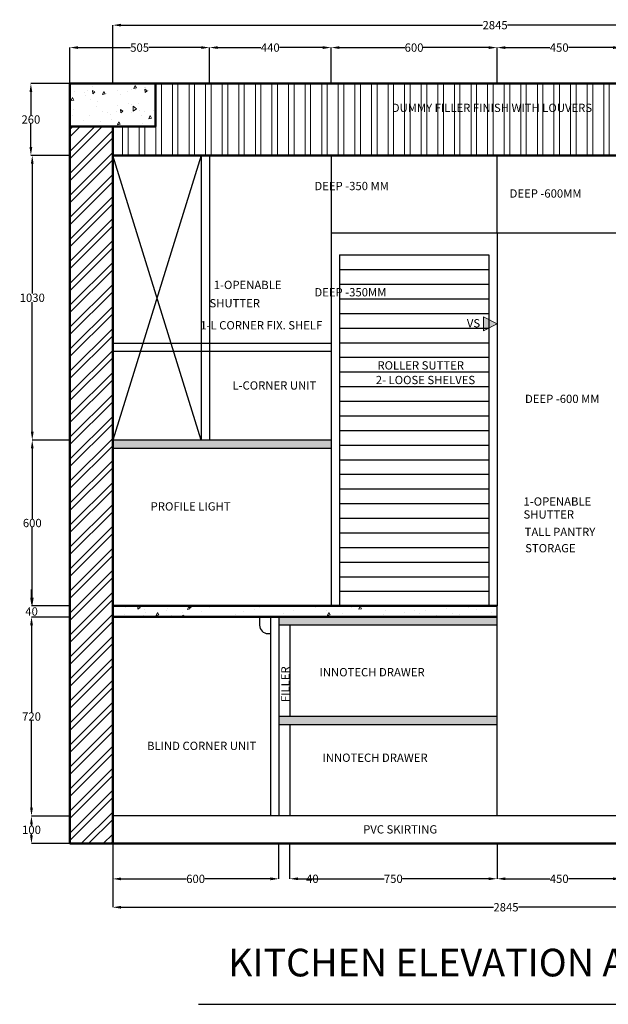
# Model space of a CAD drawing. Units: millimetres. Extents: x 26138 to 44889, y 15820 to 21179.
# Tile 7 of 8: x 41289 to 43418, y 15893 to 19455. Entities that reach past the tile are written whole.
import ezdxf

# ---------------------------------------------------------------- set-up
doc = ezdxf.new("R2010")
doc.units = ezdxf.units.MM
doc.header["$MEASUREMENT"] = 0
doc.header["$PDMODE"] = 3
for name, color, linetype, lineweight in [('A-ANNO-DIMS', 70, 'Continuous', 18), ('A-ANNO-SYMB', 1, 'Continuous', 18), ('A-ANNO-TEXT', 7, 'Continuous', 18), ('A-ELEV', 7, 'Continuous', 25), ('A-FURN-PATT', 40, 'Continuous', 13), ('A-WALL', 1, 'Continuous', 50), ('A-WALL-PATT', 8, 'Continuous', 13)]:
    doc.layers.add(name, color=color, linetype=linetype, lineweight=lineweight)
doc.styles.get("Standard").update_dxf_attribs({"font": 'arial.ttf'})
doc.dimstyles.get("Standard").update_dxf_attribs({"dimtxt": 30, "dimasz": 30, "dimexe": 0.18, "dimexo": 0.0625, "dimgap": 0.09, "dimtad": 0, "dimtih": 1, "dimtoh": 1, "dimdec": 0, "dimzin": 0, "dimdsep": 46, "dimtxsty": 'Standard', "dimcen": 0.09, "dimadec": 0, "dimazin": 0, "dimtfac": 1, "dimtdec": 0, "dimtofl": 0, "dimtmove": 0, "dimatfit": 3, "dimfxl": 1, "dimtolj": 1, "dimtzin": 0, "dimarcsym": 0})
pattern_1 = [(95, (-2438.25, -2020.09), (88.24832, 74.04913), [12, -132]), (40, (-2438.25, -2020.09), (-100.79875, 69.4029), [9.6, -105.6]), (145.45144, (-2430.9, -2013.92), (-12.55043, 143.45204), [10.19843, -112.18274]), (91.1842, (-2460.88, -1997.47), (139.47094, 102.0182), [18, -198]), (141.63564, (-2449.26, -1988.96), (-4.464, 215.95387), [15.29765, -168.2742]), (36.18416, (-2460.88, -1997.47), (-4.464, 215.95387), [14.4, -158.4]), (66, (-2443.91, -1991.81), (113.08345, 21.9812), [12, -132]), (11, (-2443.91, -1991.81), (-54.51337, 109.56935), [9.6, -105.6]), (116.45144, (-2434.49, -1989.98), (58.57008, 131.55054), [10.19843, -112.18274]), (82.5, (-2438.253, -2020.094), (-36.28691, 39.03837), [0, -104.32, 0, -107.2, 0, -106]), (52.5, (-2438.253, -2020.094), (-14.85967, 74.38551), [0, -61.12, 0, -101.92, 0, -40.4]), (12.5, (-2463.483, -2045.323), (62.946907, 57.843322), [0, -40, 0, -124.8, 0, -165.6]), (2.5, (-2474.796, -2056.64), (54.6544, 77.30557), [0, -52, 0, -82.88, 0, -117.6])]

# ---------------------------------------------------------------- blocks, each defined once
blk = doc.blocks.new('*D93')
at = {"layer": 'A-ANNO-DIMS', "color": 0, "lineweight": -2, "transparency": 16777216}
for p, q in [((41470.8, 19224.3), (41470.8, 19354.6)), ((41500.8, 19354.4), (41690, 19354.4)), ((41945.8, 19354.4), (41756.6, 19354.4)), ((41975.8, 19224.3), (41975.8, 19354.6))]:
    blk.add_line(p, q, dxfattribs=at)
at = {"layer": 'A-ANNO-DIMS', "color": 0, "transparency": 16777216}
for points in [[(41500.8, 19359.4), (41500.8, 19349.4), (41470.8, 19354.4)], [(41945.8, 19359.4), (41945.8, 19349.4), (41975.8, 19354.4)]]:
    blk.add_solid(points, dxfattribs=at)
at = {"layer": 'Defpoints', "color": 0, "transparency": 16777216}
for p in [(41975.8, 19354.4), (41470.8, 19224.2), (41975.8, 19224.2)]:
    blk.add_point(p, dxfattribs=at)
at = {"layer": 'A-ANNO-DIMS', "color": 0, "transparency": 16777216, "insert": (41723.3, 19354.4), "char_height": 30, "attachment_point": 5}
blk.add_mtext('\\A1;505', dxfattribs=at)
blk = doc.blocks.new('*D94')
at = {"layer": 'A-ANNO-DIMS', "color": 0, "lineweight": -2, "transparency": 16777216}
for p, q in [((41975.8, 19224.3), (41975.8, 19354.6)), ((42005.8, 19354.4), (42162, 19354.4)), ((42385.8, 19354.4), (42229.6, 19354.4)), ((42415.8, 19224.3), (42415.8, 19354.6))]:
    blk.add_line(p, q, dxfattribs=at)
at = {"layer": 'A-ANNO-DIMS', "color": 0, "transparency": 16777216}
for points in [[(42005.8, 19359.4), (42005.8, 19349.4), (41975.8, 19354.4)], [(42385.8, 19359.4), (42385.8, 19349.4), (42415.8, 19354.4)]]:
    blk.add_solid(points, dxfattribs=at)
at = {"layer": 'Defpoints', "color": 0, "transparency": 16777216}
for p in [(42415.8, 19354.4), (41975.8, 19224.2), (42415.8, 19224.2)]:
    blk.add_point(p, dxfattribs=at)
at = {"layer": 'A-ANNO-DIMS', "color": 0, "transparency": 16777216, "insert": (42195.8, 19354.4), "char_height": 30, "attachment_point": 5}
blk.add_mtext('\\A1;440', dxfattribs=at)
blk = doc.blocks.new('*D95')
at = {"layer": 'A-ANNO-DIMS', "color": 0, "lineweight": -2, "transparency": 16777216}
for p, q in [((42415.8, 19224.3), (42415.8, 19354.6)), ((42445.8, 19354.4), (42682.5, 19354.4)), ((42985.8, 19354.4), (42749.1, 19354.4)), ((43015.8, 19224.3), (43015.8, 19354.6))]:
    blk.add_line(p, q, dxfattribs=at)
at = {"layer": 'A-ANNO-DIMS', "color": 0, "transparency": 16777216}
for points in [[(42445.8, 19359.4), (42445.8, 19349.4), (42415.8, 19354.4)], [(42985.8, 19359.4), (42985.8, 19349.4), (43015.8, 19354.4)]]:
    blk.add_solid(points, dxfattribs=at)
at = {"layer": 'Defpoints', "color": 0, "transparency": 16777216}
for p in [(43015.8, 19354.4), (42415.8, 19224.2), (43015.8, 19224.2)]:
    blk.add_point(p, dxfattribs=at)
at = {"layer": 'A-ANNO-DIMS', "color": 0, "transparency": 16777216, "insert": (42715.8, 19354.4), "char_height": 30, "attachment_point": 5}
blk.add_mtext('\\A1;600', dxfattribs=at)
blk = doc.blocks.new('*D96')
at = {"layer": 'A-ANNO-DIMS', "color": 0, "lineweight": -2, "transparency": 16777216}
for p, q in [((43015.8, 19224.3), (43015.8, 19354.6)), ((43045.8, 19354.4), (43207, 19354.4)), ((43435.8, 19354.4), (43274.6, 19354.4)), ((43465.8, 19224.3), (43465.8, 19354.6))]:
    blk.add_line(p, q, dxfattribs=at)
at = {"layer": 'A-ANNO-DIMS', "color": 0, "transparency": 16777216}
for points in [[(43045.8, 19359.4), (43045.8, 19349.4), (43015.8, 19354.4)], [(43435.8, 19359.4), (43435.8, 19349.4), (43465.8, 19354.4)]]:
    blk.add_solid(points, dxfattribs=at)
at = {"layer": 'Defpoints', "color": 0, "transparency": 16777216}
for p in [(43465.8, 19354.4), (43015.8, 19224.2), (43465.8, 19224.2)]:
    blk.add_point(p, dxfattribs=at)
at = {"layer": 'A-ANNO-DIMS', "color": 0, "transparency": 16777216, "insert": (43240.8, 19354.4), "char_height": 30, "attachment_point": 5}
blk.add_mtext('\\A1;450', dxfattribs=at)
blk = doc.blocks.new('*D99')
at = {"layer": 'A-ANNO-DIMS', "color": 0, "lineweight": -2, "transparency": 16777216}
for p, q in [((41625.8, 19224.3), (41625.8, 19435.8)), ((41655.8, 19435.6), (42963.6, 19435.6)), ((44440.8, 19435.6), (43054.1, 19435.6)), ((44470.8, 19224.3), (44470.8, 19435.8))]:
    blk.add_line(p, q, dxfattribs=at)
at = {"layer": 'A-ANNO-DIMS', "color": 0, "transparency": 16777216}
for points in [[(41655.8, 19440.6), (41655.8, 19430.6), (41625.8, 19435.6)], [(44440.8, 19440.6), (44440.8, 19430.6), (44470.8, 19435.6)]]:
    blk.add_solid(points, dxfattribs=at)
at = {"layer": 'Defpoints', "color": 0, "transparency": 16777216}
for p in [(41625.8, 19435.6), (41625.8, 19224.2), (44470.8, 19224.2)]:
    blk.add_point(p, dxfattribs=at)
at = {"layer": 'A-ANNO-DIMS', "color": 0, "transparency": 16777216, "insert": (43008.9, 19435.6), "char_height": 30, "attachment_point": 5}
blk.add_mtext('\\A1;2845', dxfattribs=at)
blk = doc.blocks.new('*D105')
at = {"layer": 'A-ANNO-DIMS', "color": 0, "lineweight": -2, "transparency": 16777216}
for p, q in [((41625.8, 16474.2), (41625.8, 16346.6)), ((42225.8, 16474.2), (42225.8, 16346.6)), ((41655.8, 16346.7), (41892.5, 16346.7)), ((42195.8, 16346.7), (41959.1, 16346.7))]:
    blk.add_line(p, q, dxfattribs=at)
at = {"layer": 'A-ANNO-DIMS', "color": 0, "transparency": 16777216}
for points in [[(41655.8, 16351.7), (41655.8, 16341.7), (41625.8, 16346.7)], [(42195.8, 16351.7), (42195.8, 16341.7), (42225.8, 16346.7)]]:
    blk.add_solid(points, dxfattribs=at)
at = {"layer": 'Defpoints', "color": 0, "transparency": 16777216}
for p in [(41625.8, 16474.2), (42225.8, 16474.2), (42225.8, 16346.7)]:
    blk.add_point(p, dxfattribs=at)
at = {"layer": 'A-ANNO-DIMS', "color": 0, "transparency": 16777216, "insert": (41925.8, 16346.7), "char_height": 30, "attachment_point": 5}
blk.add_mtext('\\A1;600', dxfattribs=at)
blk = doc.blocks.new('*D106')
at = {"layer": 'A-ANNO-DIMS', "color": 0, "lineweight": -2, "transparency": 16777216}
for p, q in [((42225.8, 16474.2), (42225.8, 16346.9)), ((42265.8, 16474.2), (42265.8, 16346.9)), ((42195.8, 16347.1), (42165.8, 16347.1)), ((42295.8, 16347.1), (42325.8, 16347.1))]:
    blk.add_line(p, q, dxfattribs=at)
at = {"layer": 'A-ANNO-DIMS', "color": 0, "transparency": 16777216}
for points in [[(42195.8, 16352.1), (42195.8, 16342.1), (42225.8, 16347.1)], [(42295.8, 16352.1), (42295.8, 16342.1), (42265.8, 16347.1)]]:
    blk.add_solid(points, dxfattribs=at)
at = {"layer": 'Defpoints', "color": 0, "transparency": 16777216}
for p in [(42225.8, 16474.2), (42265.8, 16474.2), (42265.8, 16347.1)]:
    blk.add_point(p, dxfattribs=at)
at = {"layer": 'A-ANNO-DIMS', "color": 0, "transparency": 16777216, "insert": (42347.9, 16347.1), "char_height": 30, "attachment_point": 5}
blk.add_mtext('\\A1;40', dxfattribs=at)
blk = doc.blocks.new('*D107')
at = {"layer": 'A-ANNO-DIMS', "color": 0, "lineweight": -2, "transparency": 16777216}
for p, q in [((42265.8, 16474.2), (42265.8, 16346.9)), ((43015.8, 16474.2), (43015.8, 16346.9)), ((42295.8, 16347.1), (42607.7, 16347.1)), ((42985.8, 16347.1), (42673.9, 16347.1))]:
    blk.add_line(p, q, dxfattribs=at)
at = {"layer": 'A-ANNO-DIMS', "color": 0, "transparency": 16777216}
for points in [[(42295.8, 16352.1), (42295.8, 16342.1), (42265.8, 16347.1)], [(42985.8, 16352.1), (42985.8, 16342.1), (43015.8, 16347.1)]]:
    blk.add_solid(points, dxfattribs=at)
at = {"layer": 'Defpoints', "color": 0, "transparency": 16777216}
for p in [(42265.8, 16474.2), (43015.8, 16474.2), (43015.8, 16347.1)]:
    blk.add_point(p, dxfattribs=at)
at = {"layer": 'A-ANNO-DIMS', "color": 0, "transparency": 16777216, "insert": (42640.8, 16347.1), "char_height": 30, "attachment_point": 5}
blk.add_mtext('\\A1;750', dxfattribs=at)
blk = doc.blocks.new('*D108')
at = {"layer": 'A-ANNO-DIMS', "color": 0, "lineweight": -2, "transparency": 16777216}
for p, q in [((43015.8, 16474.2), (43015.8, 16346.9)), ((43465.8, 16474.2), (43465.8, 16346.9)), ((43045.8, 16347.1), (43207, 16347.1)), ((43435.8, 16347.1), (43274.6, 16347.1))]:
    blk.add_line(p, q, dxfattribs=at)
at = {"layer": 'A-ANNO-DIMS', "color": 0, "transparency": 16777216}
for points in [[(43045.8, 16352.1), (43045.8, 16342.1), (43015.8, 16347.1)], [(43435.8, 16352.1), (43435.8, 16342.1), (43465.8, 16347.1)]]:
    blk.add_solid(points, dxfattribs=at)
at = {"layer": 'Defpoints', "color": 0, "transparency": 16777216}
for p in [(43015.8, 16474.2), (43465.8, 16474.2), (43465.8, 16347.1)]:
    blk.add_point(p, dxfattribs=at)
at = {"layer": 'A-ANNO-DIMS', "color": 0, "transparency": 16777216, "insert": (43240.8, 16347.1), "char_height": 30, "attachment_point": 5}
blk.add_mtext('\\A1;450', dxfattribs=at)
blk = doc.blocks.new('*D110')
at = {"layer": 'A-ANNO-DIMS', "color": 0, "lineweight": -2, "transparency": 16777216}
for p, q in [((41470.7, 19224.2), (41329.7, 19224.2)), ((41329.9, 19194.2), (41329.9, 19109.6)), ((41329.9, 18994.2), (41329.9, 19078.8)), ((41470.7, 18964.2), (41329.7, 18964.2))]:
    blk.add_line(p, q, dxfattribs=at)
at = {"layer": 'A-ANNO-DIMS', "color": 0, "transparency": 16777216}
for points in [[(41324.9, 19194.2), (41334.9, 19194.2), (41329.9, 19224.2)], [(41324.9, 18994.2), (41334.9, 18994.2), (41329.9, 18964.2)]]:
    blk.add_solid(points, dxfattribs=at)
at = {"layer": 'Defpoints', "color": 0, "transparency": 16777216}
for p in [(41470.8, 19224.2), (41329.9, 18964.2), (41470.8, 18964.2)]:
    blk.add_point(p, dxfattribs=at)
at = {"layer": 'A-ANNO-DIMS', "color": 0, "transparency": 16777216, "insert": (41329.9, 19094.2), "char_height": 30, "attachment_point": 5}
blk.add_mtext('\\A1;260', dxfattribs=at)
blk = doc.blocks.new('*D111')
at = {"layer": 'A-ANNO-DIMS', "color": 0, "lineweight": -2, "transparency": 16777216}
for p, q in [((41470.7, 18964.2), (41334.7, 18964.2)), ((41334.9, 18934.2), (41334.9, 18464.7)), ((41334.9, 17964.2), (41334.9, 18433.8)), ((41470.7, 17934.2), (41334.7, 17934.2))]:
    blk.add_line(p, q, dxfattribs=at)
at = {"layer": 'A-ANNO-DIMS', "color": 0, "transparency": 16777216}
for points in [[(41329.9, 18934.2), (41339.9, 18934.2), (41334.9, 18964.2)], [(41329.9, 17964.2), (41339.9, 17964.2), (41334.9, 17934.2)]]:
    blk.add_solid(points, dxfattribs=at)
at = {"layer": 'Defpoints', "color": 0, "transparency": 16777216}
for p in [(41470.8, 18964.2), (41334.9, 17934.2), (41470.8, 17934.2)]:
    blk.add_point(p, dxfattribs=at)
at = {"layer": 'A-ANNO-DIMS', "color": 0, "transparency": 16777216, "insert": (41334.9, 18449.2), "char_height": 30, "attachment_point": 5}
blk.add_mtext('\\A1;1030', dxfattribs=at)
blk = doc.blocks.new('*D112')
at = {"layer": 'A-ANNO-DIMS', "color": 0, "lineweight": -2, "transparency": 16777216}
for p, q in [((41470.7, 17934.2), (41334.7, 17934.2)), ((41334.9, 17904.2), (41334.9, 17649.6)), ((41334.9, 17364.2), (41334.9, 17618.8)), ((41470.7, 17334.2), (41334.7, 17334.2))]:
    blk.add_line(p, q, dxfattribs=at)
at = {"layer": 'A-ANNO-DIMS', "color": 0, "transparency": 16777216}
for points in [[(41329.9, 17904.2), (41339.9, 17904.2), (41334.9, 17934.2)], [(41329.9, 17364.2), (41339.9, 17364.2), (41334.9, 17334.2)]]:
    blk.add_solid(points, dxfattribs=at)
at = {"layer": 'Defpoints', "color": 0, "transparency": 16777216}
for p in [(41470.8, 17934.2), (41334.9, 17334.2), (41470.8, 17334.2)]:
    blk.add_point(p, dxfattribs=at)
at = {"layer": 'A-ANNO-DIMS', "color": 0, "transparency": 16777216, "insert": (41334.9, 17634.2), "char_height": 30, "attachment_point": 5}
blk.add_mtext('\\A1;600', dxfattribs=at)
blk = doc.blocks.new('*D113')
at = {"layer": 'A-ANNO-DIMS', "color": 0, "lineweight": -2, "transparency": 16777216}
for p, q in [((41332.4, 17364.2), (41332.4, 17394.2)), ((41470.7, 17334.2), (41332.2, 17334.2)), ((41470.7, 17294.2), (41332.2, 17294.2)), ((41332.4, 17264.2), (41332.4, 17234.2))]:
    blk.add_line(p, q, dxfattribs=at)
at = {"layer": 'A-ANNO-DIMS', "color": 0, "transparency": 16777216}
for points in [[(41327.4, 17364.2), (41337.4, 17364.2), (41332.4, 17334.2)], [(41327.4, 17264.2), (41337.4, 17264.2), (41332.4, 17294.2)]]:
    blk.add_solid(points, dxfattribs=at)
at = {"layer": 'Defpoints', "color": 0, "transparency": 16777216}
for p in [(41470.8, 17334.2), (41332.4, 17294.2), (41470.8, 17294.2)]:
    blk.add_point(p, dxfattribs=at)
at = {"layer": 'A-ANNO-DIMS', "color": 0, "transparency": 16777216, "insert": (41332.4, 17314.2), "char_height": 30, "attachment_point": 5}
blk.add_mtext('\\A1;40', dxfattribs=at)
blk = doc.blocks.new('*D114')
at = {"layer": 'A-ANNO-DIMS', "color": 0, "lineweight": -2, "transparency": 16777216}
for p, q in [((41470.7, 17294.2), (41332, 17294.2)), ((41332.2, 17264.2), (41332.2, 16949.6)), ((41332.2, 16604.2), (41332.2, 16918.8)), ((41470.7, 16574.2), (41332, 16574.2))]:
    blk.add_line(p, q, dxfattribs=at)
at = {"layer": 'A-ANNO-DIMS', "color": 0, "transparency": 16777216}
for points in [[(41327.2, 17264.2), (41337.2, 17264.2), (41332.2, 17294.2)], [(41327.2, 16604.2), (41337.2, 16604.2), (41332.2, 16574.2)]]:
    blk.add_solid(points, dxfattribs=at)
at = {"layer": 'Defpoints', "color": 0, "transparency": 16777216}
for p in [(41470.8, 17294.2), (41332.2, 16574.2), (41470.8, 16574.2)]:
    blk.add_point(p, dxfattribs=at)
at = {"layer": 'A-ANNO-DIMS', "color": 0, "transparency": 16777216, "insert": (41332.2, 16934.2), "char_height": 30, "attachment_point": 5}
blk.add_mtext('\\A1;720', dxfattribs=at)
blk = doc.blocks.new('*D115')
at = {"layer": 'A-ANNO-DIMS', "color": 0, "lineweight": -2, "transparency": 16777216}
for p, q in [((41470.7, 16574.2), (41331.8, 16574.2)), ((41332, 16544.2), (41332, 16539.6)), ((41332, 16504.2), (41332, 16508.8)), ((41470.7, 16474.2), (41331.8, 16474.2))]:
    blk.add_line(p, q, dxfattribs=at)
at = {"layer": 'A-ANNO-DIMS', "color": 0, "transparency": 16777216}
for points in [[(41327, 16544.2), (41337, 16544.2), (41332, 16574.2)], [(41327, 16504.2), (41337, 16504.2), (41332, 16474.2)]]:
    blk.add_solid(points, dxfattribs=at)
at = {"layer": 'Defpoints', "color": 0, "transparency": 16777216}
for p in [(41470.8, 16574.2), (41332, 16474.2), (41470.8, 16474.2)]:
    blk.add_point(p, dxfattribs=at)
at = {"layer": 'A-ANNO-DIMS', "color": 0, "transparency": 16777216, "insert": (41332, 16524.2), "char_height": 30, "attachment_point": 5}
blk.add_mtext('\\A1;100', dxfattribs=at)
blk = doc.blocks.new('*D116')
at = {"layer": 'A-ANNO-DIMS', "color": 0, "lineweight": -2, "transparency": 16777216}
for p, q in [((41625.8, 16474.2), (41625.8, 16243.8)), ((44470.8, 16474.2), (44470.8, 16243.8)), ((41655.8, 16244), (43003, 16244)), ((44440.8, 16244), (43093.5, 16244))]:
    blk.add_line(p, q, dxfattribs=at)
at = {"layer": 'A-ANNO-DIMS', "color": 0, "transparency": 16777216}
for points in [[(41655.8, 16249), (41655.8, 16239), (41625.8, 16244)], [(44440.8, 16249), (44440.8, 16239), (44470.8, 16244)]]:
    blk.add_solid(points, dxfattribs=at)
at = {"layer": 'Defpoints', "color": 0, "transparency": 16777216}
for p in [(41625.8, 16474.2), (44470.8, 16474.2), (44470.8, 16244)]:
    blk.add_point(p, dxfattribs=at)
at = {"layer": 'A-ANNO-DIMS', "color": 0, "transparency": 16777216, "insert": (43048.3, 16244), "char_height": 30, "attachment_point": 5}
blk.add_mtext('\\A1;2845', dxfattribs=at)
blk = doc.blocks.new('SYMB-VS-TRIANGLE')
for p, q in [((0, 0), (25, 49.1)), ((50, 0), (25, 49.1)), ((0, 0), (50, 0))]:
    blk.add_line(p, q)

msp = doc.modelspace()

# ---------------------------------------------------------------- hatches: boundary and pattern name
at = {"layer": 'A-FURN-PATT'}
h = msp.add_hatch(color=256, dxfattribs=at)
h.dxf.hatch_style = 1
h.paths.add_polyline_path([(42966.733, 18330.058), (42966.733, 18380.058), (43015.825, 18355.058)])
h = msp.add_hatch(color=256, dxfattribs=at)
h.dxf.hatch_style = 1
h.paths.add_polyline_path([(42415.796, 17904.233), (42415.796, 17934.233), (41625.796, 17934.233), (41625.796, 17904.233)])
h = msp.add_hatch(color=256, dxfattribs=at)
h.dxf.hatch_style = 1
h.paths.add_polyline_path([(42227.534, 17294.233), (42227.534, 17264.233), (43015.796, 17264.233), (43015.796, 17294.233)])
h = msp.add_hatch(color=256, dxfattribs=at)
h.dxf.hatch_style = 1
h.paths.add_polyline_path([(43015.796, 16904.233), (43015.796, 16934.233), (42227.534, 16934.233), (42227.534, 16904.233)])
at = {"layer": 'A-WALL-PATT'}
h = msp.add_hatch(dxfattribs=at)
h.set_pattern_fill('AR-CONC', color=256, scale=16, angle=45)
h.set_pattern_definition(pattern_1)
h.paths.add_polyline_path([(41780.796, 19224.233), (41470.796, 19224.233), (41470.796, 19069.233), (41780.796, 19069.233)])
h = msp.add_hatch(dxfattribs=at)
h.set_pattern_fill('ANSI32', color=256, scale=160, angle=45)
h.set_pattern_definition([(90, (-2438.25, -2020.094), (-60, 0), []), (90, (-2418.25, -2000.094), (-60, 0), [])])
h.paths.add_polyline_path([(44315.796, 18964.233), (44315.796, 19224.233), (41780.796, 19224.233), (41780.796, 19069.233), (41625.796, 19069.233), (41625.796, 18964.233)])
h.paths.add_polyline_path([(42627.517, 19113.099), (43434.744, 19113.099), (43434.744, 19159.664), (42627.517, 19159.664)], flags=24)
h = msp.add_hatch(dxfattribs=at)
h.set_pattern_fill('ANSI32', color=256, scale=150)
h.set_pattern_definition([(45, (-2438.253, -2020.094), (-39.774756, 39.774756), []), (45, (-2411.736, -2020.094), (-39.774756, 39.774756), [])])
h.paths.add_polyline_path([(41470.796, 16474.233), (41625.796, 16474.233), (41625.796, 19069.233), (41470.796, 19069.233)])
h = msp.add_hatch(dxfattribs=at)
h.set_pattern_fill('AR-CONC', color=256, scale=16, angle=45)
h.set_pattern_definition(pattern_1)
h.paths.add_polyline_path([(41625.796, 17334.233), (41625.796, 17294.233), (42227.534, 17294.233), (43015.796, 17294.233), (43015.796, 17334.233)])

# ---------------------------------------------------------------- linework, layer by layer
at = {"layer": 'A-ELEV'}
for p, q in [((41945.796, 18964.233), (41625.796, 17934.233)), ((41945.796, 17934.233), (41625.796, 18964.233)), ((41945.796, 18964.233), (41945.796, 17934.233)), ((41975.796, 18964.233), (41975.796, 17934.233)), ((42415.796, 18964.233), (42415.796, 17334.233)), ((43015.796, 18684.233), (43015.796, 18964.233)), ((42415.796, 18684.233), (43015.796, 18684.233)), ((43015.796, 18684.233), (43015.796, 17334.233)), ((43015.796, 18684.233), (44470.796, 18684.233)), ((42445.796, 18604.233), (42985.796, 18604.233)), ((42445.796, 18604.233), (42445.796, 17334.233)), ((42985.796, 18604.233), (42985.796, 17334.233)), ((42445.796, 18551.316), (42985.796, 18551.316)), ((42445.796, 18498.399), (42985.796, 18498.399)), ((42445.796, 18445.483), (42985.796, 18445.483)), ((42445.796, 18392.566), (42985.796, 18392.566)), ((42445.796, 18339.649), (42985.796, 18339.649)), ((42415.796, 18284.233), (41625.796, 18284.233)), ((42445.796, 18286.733), (42985.796, 18286.733)), ((42415.796, 18254.233), (41625.796, 18254.233)), ((42445.796, 18233.816), (42985.796, 18233.816)), ((42445.796, 18180.899), (42985.796, 18180.899)), ((42445.796, 18127.983), (42985.796, 18127.983)), ((42445.796, 18075.066), (42985.796, 18075.066)), ((42445.796, 18022.149), (42985.796, 18022.149)), ((42445.796, 17969.233), (42985.796, 17969.233)), ((42415.796, 17934.233), (41625.796, 17934.233)), ((42415.796, 17904.233), (41625.796, 17904.233)), ((42445.796, 17916.316), (42985.796, 17916.316)), ((42445.796, 17863.399), (42985.796, 17863.399)), ((42445.796, 17810.483), (42985.796, 17810.483)), ((42445.796, 17757.566), (42985.796, 17757.566)), ((42445.796, 17704.649), (42985.796, 17704.649)), ((42445.796, 17651.733), (42985.796, 17651.733)), ((42445.796, 17598.816), (42985.796, 17598.816)), ((42445.796, 17545.899), (42985.796, 17545.899)), ((42445.796, 17492.983), (42985.796, 17492.983)), ((42445.796, 17440.066), (42985.796, 17440.066)), ((42445.796, 17387.149), (42985.796, 17387.149)), ((43015.796, 16574.233), (43015.796, 17334.233)), ((42157.268, 17294.233), (42157.268, 17264.313)), ((42197.534, 16574.233), (42197.534, 17294.233)), ((42227.534, 16574.233), (42227.534, 17294.233)), ((43015.796, 17264.233), (42227.534, 17264.233)), ((42267.534, 16934.233), (42267.534, 17264.233)), ((42187.268, 17234.313), (42197.534, 17234.313)), ((43015.796, 16934.233), (42227.534, 16934.233)), ((43015.796, 16904.233), (42227.534, 16904.233)), ((42267.534, 16574.233), (42267.534, 16904.233)), ((43465.796, 16574.233), (41625.796, 16574.233)), ((41936.11, 15892.9), (43949.787, 15892.9))]:
    msp.add_line(p, q, dxfattribs=at)
msp.add_arc((42187.268, 17264.313), 30, 180, 270, dxfattribs=at)
at = {"layer": 'A-WALL'}
for p, q in [((41470.796, 19224.233), (44470.796, 19224.233)), ((41470.796, 16474.233), (41470.796, 19224.233)), ((41780.796, 19069.233), (41780.796, 19224.233)), ((41470.796, 19069.233), (41780.796, 19069.233)), ((41625.796, 16474.233), (41625.796, 19069.233)), ((44470.796, 18964.233), (41625.796, 18964.233)), ((43015.796, 17334.233), (41625.796, 17334.233)), ((42227.534, 17294.233), (41625.796, 17294.233)), ((43015.796, 17294.233), (42227.534, 17294.233)), ((44470.796, 16474.233), (41470.796, 16474.233))]:
    msp.add_line(p, q, dxfattribs=at)

# ---------------------------------------------------------------- block references
at = {"layer": 'A-ANNO-SYMB', "rotation": 270.0000000000064}
msp.add_blockref('SYMB-VS-TRIANGLE', (42966.733, 18380.058), dxfattribs=at)

# ---------------------------------------------------------------- texts
at = {"layer": 'A-ANNO-TEXT'}
for s, height, p in [('DUMMY FILLER FINISH WITH LOUVERS', 30, (42635.278, 19121.372)), ('DEEP -350 MM ', 30, (42355.459, 18838.519)), ('DEEP -600MM', 30, (43061.318, 18811.537)), ('1-OPENABLE', 30, (41991.374, 18480.694)), ('DEEP -350MM', 30, (42355.459, 18454.19)), ('SHUTTER', 30, (41975.796, 18414.532)), ('1-L CORNER FIX. SHELF', 30, (41942.692, 18334.748)), ('VS', 30, (42906.8, 18341.842)), ('ROLLER SUTTER ', 30, (42583.307, 18189.607)), ('L-CORNER UNIT', 30, (42059.055, 18116.873)), ('2- LOOSE SHELVES', 30, (42577.425, 18136.69)), ('DEEP -600 MM', 30, (43117.049, 18068.4)), ('PROFILE LIGHT', 30, (41763.06, 17679.343)), ('1-OPENABLE ', 30, (43111.615, 17697.035)), ('SHUTTER', 30, (43111.615, 17650.238)), ('TALL PANTRY', 30, (43115.687, 17587.164)), ('STORAGE', 30, (43117.723, 17528.16)), ('INNOTECH DRAWER', 30, (42373.808, 17079.461)), ('BLIND CORNER UNIT', 30, (41750.112, 16812.978)), ('INNOTECH DRAWER', 30, (42384.557, 16770.088)), ('PVC SKIRTING', 30, (42531.604, 16510.774)), ('KITCHEN ELEVATION AT-C', 100, (42043.106, 15993.854))]:
    msp.add_text(s, height=height, dxfattribs=at).set_placement(p)
msp.add_text('FILLER', height=30, rotation=90, dxfattribs=at).set_placement((42265.232, 16986.501))

# ---------------------------------------------------------------- dimensions: what is measured, and where the dimension line sits
at = {"layer": 'A-ANNO-DIMS'}
for base, p1, p2, picture, middle in [((41625.796, 19435.636), (44470.796, 19224.233), (41625.796, 19224.233), '*D99', (43008.876, 19435.636)), ((44470.796, 16244.003), (41625.796, 16474.233), (44470.796, 16474.233), '*D116', (43048.296, 16244.003))]:
    dim = msp.add_linear_dim(base=base, p1=p1, p2=p2, dimstyle='Standard', override={"dimclrd": 0, "dimclre": 0, "dimclrt": 0}, dxfattribs=at)
    dim.commit()
    dim.dimension.update_dxf_attribs({"geometry": picture, "text_midpoint": middle, "dimtype": 160})
for base, p1, p2, picture, middle in [((41975.796, 19354.4), (41470.796, 19224.233), (41975.796, 19224.233), '*D93', (41723.296, 19354.4)), ((42415.796, 19354.4), (41975.796, 19224.233), (42415.796, 19224.233), '*D94', (42195.796, 19354.4)), ((43015.796, 19354.4), (42415.796, 19224.233), (43015.796, 19224.233), '*D95', (42715.796, 19354.4)), ((43465.796, 19354.4), (43015.796, 19224.233), (43465.796, 19224.233), '*D96', (43240.796, 19354.4)), ((42225.796, 16346.739), (41625.796, 16474.233), (42225.796, 16474.233), '*D105', (41925.796, 16346.739)), ((42265.796, 16347.119), (42225.796, 16474.233), (42265.796, 16474.233), '*D106', (42347.925, 16347.119)), ((43015.796, 16347.119), (42265.796, 16474.233), (43015.796, 16474.233), '*D107', (42640.796, 16347.119)), ((43465.796, 16347.119), (43015.796, 16474.233), (43465.796, 16474.233), '*D108', (43240.796, 16347.119))]:
    dim = msp.add_linear_dim(base=base, p1=p1, p2=p2, dimstyle='Standard', override={"dimclrd": 0, "dimclre": 0, "dimclrt": 0}, dxfattribs=at)
    dim.commit()
    dim.dimension.update_dxf_attribs({"geometry": picture, "text_midpoint": middle})
for base, p1, p2, picture, middle in [((41329.883, 18964.233), (41470.796, 19224.233), (41470.796, 18964.233), '*D110', (41329.883, 19094.233)), ((41334.883, 17934.233), (41470.796, 18964.233), (41470.796, 17934.233), '*D111', (41334.883, 18449.233)), ((41334.883, 17334.233), (41470.796, 17934.233), (41470.796, 17334.233), '*D112', (41334.883, 17634.233)), ((41332.383, 17294.233), (41470.796, 17334.233), (41470.796, 17294.233), '*D113', (41332.383, 17314.233)), ((41332.203, 16574.233), (41470.796, 17294.233), (41470.796, 16574.233), '*D114', (41332.203, 16934.233)), ((41332.023, 16474.233), (41470.796, 16574.233), (41470.796, 16474.233), '*D115', (41332.023, 16524.233))]:
    dim = msp.add_linear_dim(base=base, p1=p1, p2=p2, angle=90, dimstyle='Standard', override={"dimclrd": 0, "dimclre": 0, "dimclrt": 0}, dxfattribs=at)
    dim.commit()
    dim.dimension.update_dxf_attribs({"geometry": picture, "text_midpoint": middle})

doc.saveas('drawing.dxf')
